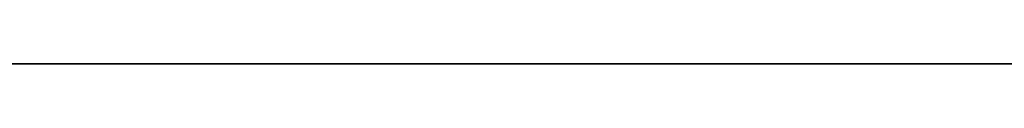
# Model space of a CAD drawing. Units: inches. Extents: x 2091 to 2899, y 967 to 2217.
# Tile 162 of 256: x 2203.142047 to 2203.143245, y 1152.24706 to 1152.24706. Entities that reach past the tile are written whole.
import ezdxf

# ---------------------------------------------------------------- set-up
doc = ezdxf.new("R2010")
doc.units = ezdxf.units.IN
doc.layers.add('A-ANNO-DIMS', color=2, linetype='Continuous', lineweight=18)
doc.layers.add('A-GLAZ', color=4, linetype='Continuous', lineweight=18)
doc.styles.get("Standard").update_dxf_attribs({"font": 'arial.ttf'})
doc.dimstyles.new('ISO-25', dxfattribs={"dimtxt": 4, "dimasz": 4, "dimexe": 1.25, "dimexo": 0.625, "dimtad": 1, "dimdec": 0, "dimlunit": 3, "dimtxsty": 'Standard', "dimcen": 2.5, "dimadec": 0, "dimazin": 0, "dimtfac": 1, "dimtdec": 0, "dimtmove": 0, "dimatfit": 3, "dimfxl": 1, "dimarcsym": 0})

# ---------------------------------------------------------------- blocks, each defined once
blk = doc.blocks.new('WIN-DOUBLE-LINE')
blk.add_line((9.1602885, -0.0004451), (0.0003982, -0.0004451))
blk = doc.blocks.new('*D91')
at = {"layer": 'A-ANNO-DIMS', "color": 0, "lineweight": -2, "transparency": 16777216}
for p, q in [((2211.650633, 1152.24706), (2098.311334, 1152.24706)), ((2099.561334, 1103.919059), (2099.561334, 1148.24706)), ((2211.518603, 1099.919059), (2098.311334, 1099.919059))]:
    blk.add_line(p, q, dxfattribs=at)
at = {"layer": 'A-ANNO-DIMS', "color": 0, "transparency": 16777216}
for points in [[(2098.8946673, 1148.24706), (2100.2280007, 1148.24706), (2099.561334, 1152.24706)], [(2098.8946673, 1103.919059), (2100.2280007, 1103.919059), (2099.561334, 1099.919059)]]:
    blk.add_solid(points, dxfattribs=at)
at = {"layer": 'Defpoints', "color": 0, "transparency": 16777216}
for p in [(2099.561334, 1152.24706), (2212.275633, 1152.24706), (2212.143603, 1099.919059)]:
    blk.add_point(p, dxfattribs=at)
at = {"layer": 'A-ANNO-DIMS', "color": 0, "transparency": 16777216, "insert": (2096.8681212, 1126.0830595), "char_height": 4, "attachment_point": 5, "rotation": 90}
blk.add_mtext('4\'-4 1/2"', dxfattribs=at)

msp = doc.modelspace()

# ---------------------------------------------------------------- block references
at = {"layer": 'A-GLAZ'}
msp.add_blockref('WIN-DOUBLE-LINE', (2203.1153443, 1152.2475047), dxfattribs=at)

# ---------------------------------------------------------------- dimensions: what is measured, and where the dimension line sits
at = {"layer": 'A-ANNO-DIMS'}
dim = msp.add_linear_dim(base=(2099.561334, 1152.24706), p1=(2212.143603, 1099.919059), p2=(2212.275633, 1152.24706), angle=90, dimstyle='ISO-25', override={"dimdec": 1, "dimlfac": 1, "dimrnd": 0, "dimzin": 1, "dimdsep": 46, "dimlunit": 4, "dimfrac": 2}, dxfattribs=at)
dim.commit()
dim.dimension.update_dxf_attribs({"geometry": '*D91', "text_midpoint": (2096.8681212, 1126.0830595)})

doc.saveas('drawing.dxf')
